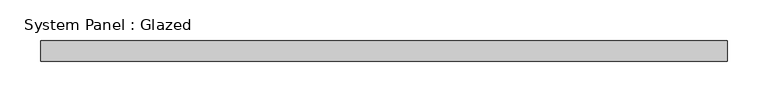
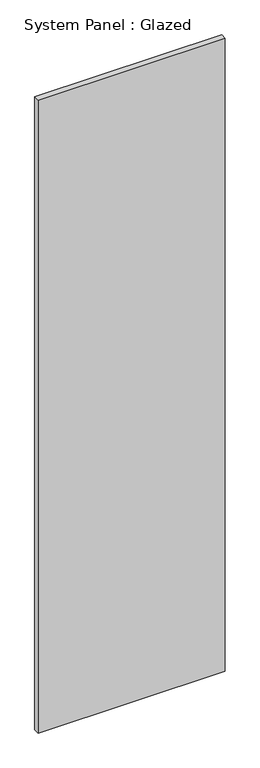
"""IFC4 building model written with IfcOpenShell, lengths in millimetres: plate geometry, System Panel : Glazed."""

from ifc_helpers import new_model, si_unit, origin, origin_with_axes, place, context, project, spatial, polyline, outline, extrude, source, transform, mapped, element, save


def system_panel_glazed_cb88c06f(model_context):
    return source(origin(), model_context, "Body", "SweptSolid", [
        extrude(outline(polyline([(419.4174419, 24.5), (-419.4174419, 24.5), (-419.4174419, 49.5), (419.4174419, 49.5), (419.4174419, 24.5)])), origin_with_axes(), (0.0, 0.0, 1.0), 3000.0),
    ])


if __name__ == "__main__":
    model = new_model("IFC4")
    model_context = context("Model", 3, world=origin())
    ifc_project = project(units=[si_unit("LENGTHUNIT", "METRE", prefix="MILLI")], contexts=[model_context])
    site = spatial("IfcSite", under=ifc_project)
    building = spatial("IfcBuilding", under=site)
    placement = place(None, origin())
    system_panel_glazed_shape = system_panel_glazed_cb88c06f(model_context)
    element("IfcPlate", 1, ObjectType="System Panel : Glazed", at=placement, inside=building, context=model_context, shape_type="MappedRepresentation", body=[
        mapped(system_panel_glazed_shape, transform((0.0, 0.0, 0.0), x_axis=(1.0, 0.0, 0.0), y_axis=(0.0, 1.0, 0.0), z_axis=(0.0, 0.0, 1.0))),
    ])
    save(model, "model.ifc")

# Revit data of these elements
# Type "System Panel : Glazed"
#   Keynote = "H11"
#   Construction Type Id = "GSP4R"
#   Analytic Construction = "1/8 in Pilkington single glazing"
#   Visual Light Transmittance = 0.9
#   Solar Heat Gain Coefficient = 0.86
#   Heat Transfer Coefficient (U) = 6.7069 W/(m²·K)
#   Define Thermal Properties by = 1
# Element 1 (IfcPlate, "System Panel : Glazed")
#   Materials on its faces: "Glass"
# Materials
#   "Glass": class "Glass", colour RGB 0 128 192, transparency 0.9, Description = "Soda Lime Glass", Cost = 0
